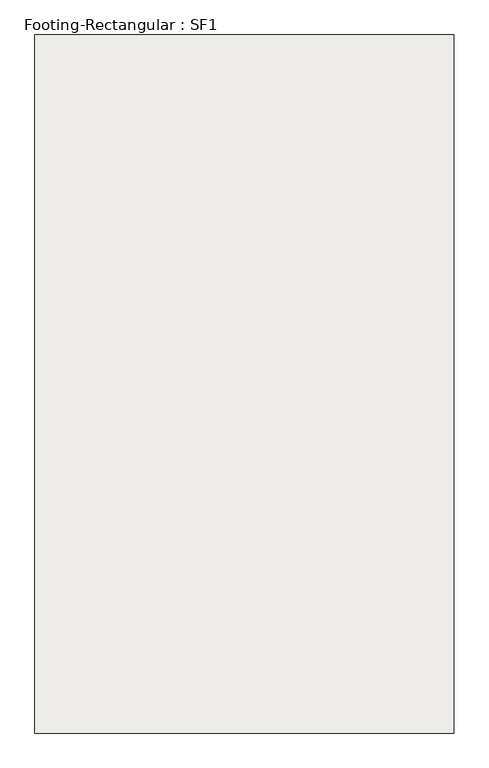
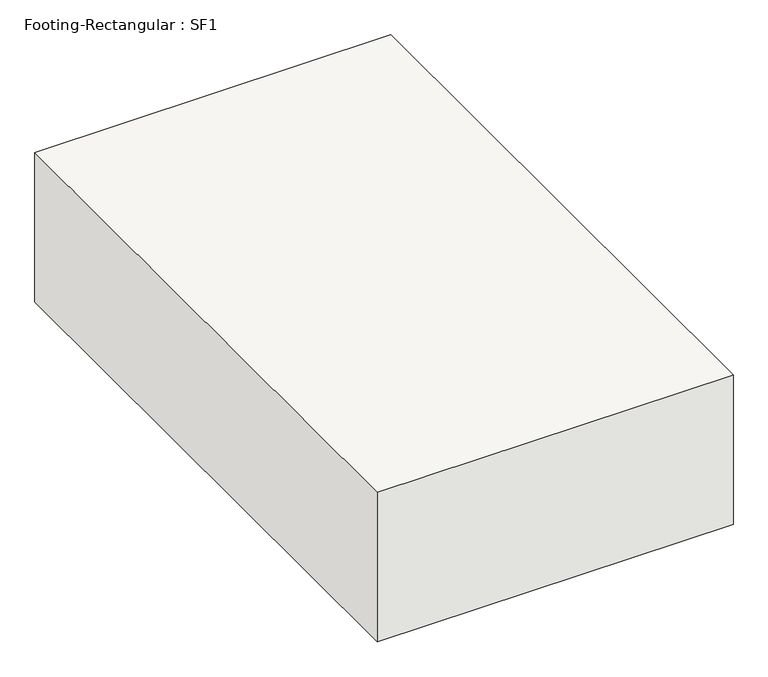
"""IFC4 building model written with IfcOpenShell, lengths in millimetres: slab geometry, Footing-Rectangular : SF1."""

from ifc_helpers import new_model, si_unit, frame, origin, place, context, project, spatial, polyline, outline, extrude, source, transform, mapped, element, save


def footing_rectangular_sf1_7ce3103a(model_context):
    return source(origin(), model_context, "Body", "SweptSolid", [
        extrude(outline(polyline([(685.8, 1143.0), (685.8, -1143.0), (-685.8, -1143.0), (-685.8, 1143.0), (685.8, 1143.0)])), frame((0.0, 0.0, -609.6), z_axis=(0.0, 0.0, 1.0), x_axis=(1.0, 0.0, 0.0)), (0.0, 0.0, 1.0), 609.6),
    ])


if __name__ == "__main__":
    model = new_model("IFC4")
    model_context = context("Model", 3, world=origin())
    ifc_project = project(units=[si_unit("LENGTHUNIT", "METRE", prefix="MILLI")], contexts=[model_context])
    site = spatial("IfcSite", under=ifc_project)
    building = spatial("IfcBuilding", under=site)
    placement = place(None, origin())
    footing_rectangular_sf1_shape = footing_rectangular_sf1_7ce3103a(model_context)
    element("IfcSlab", 1, ObjectType="Footing-Rectangular : SF1", at=placement, inside=building, context=model_context, shape_type="MappedRepresentation", body=[
        mapped(footing_rectangular_sf1_shape, transform((0.0, 0.0, 0.0), x_axis=(1.0, 0.0, 0.0), y_axis=(0.0, 1.0, 0.0), z_axis=(0.0, 0.0, 1.0))),
    ])
    save(model, "model.ifc")

# Revit data of these elements
# Type "Footing-Rectangular : SF1"
#   Width = 1371.6 mm
#   Length = 2286 mm
#   Foundation Thickness = 609.6 mm
#   Structural Material [instance default] = Concrete - Cast-in-Place Concrete
#   Assembly Code = ""
# Element 1 (IfcSlab, "Footing-Rectangular : SF1")
#   Materials on its faces: "Concrete - Cast-in-Place Concrete"
# Materials
#   "Concrete - Cast-in-Place Concrete": class "Concrete", colour RGB 192 192 192, transparency 0, Cost = 0
